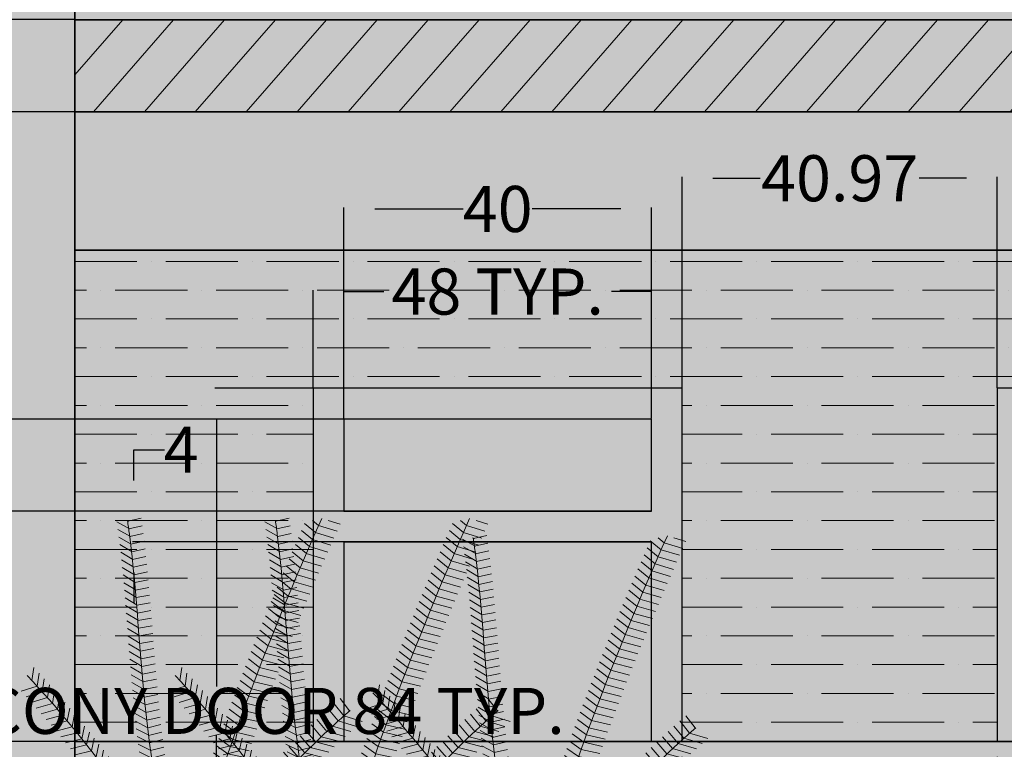
# Model space of a CAD drawing. Units: inches. Extents: x 184 to 649, y 215 to 818.
# Tile 6 of 9: x 254 to 382, y 548 to 643. Entities that reach past the tile are written whole.
import ezdxf

# ---------------------------------------------------------------- set-up
doc = ezdxf.new("R2010")
doc.units = ezdxf.units.IN
doc.header["$MEASUREMENT"] = 0
for name, color, linetype, lineweight in [('A-ANNO-DIMS', 2, 'Continuous', 18), ('A-DOOR', 4, 'Continuous', 25), ('A-ELEV', 7, 'Continuous', 35), ('A-ELEV-FILL', 9, 'Continuous', 13), ('A-ELEV-PATT', 8, 'Continuous', 13), ('L-PLNT', 84, 'Continuous', 13)]:
    doc.layers.add(name, color=color, linetype=linetype, lineweight=lineweight)
doc.styles.get("Standard").update_dxf_attribs({"font": 'arial.ttf'})
doc.dimstyles.get("Standard").update_dxf_attribs({"dimtxt": 6, "dimasz": 4, "dimexe": 0.18, "dimexo": 0.0625, "dimgap": 0.09, "dimtad": 0, "dimtih": 1, "dimtoh": 1, "dimdec": 0, "dimzin": 0, "dimdsep": 46, "dimlunit": 3, "dimtxsty": 'Standard', "dimcen": 0.09, "dimadec": 0, "dimazin": 0, "dimtfac": 1, "dimtdec": 0, "dimtofl": 0, "dimtmove": 0, "dimatfit": 3, "dimfxl": 1, "dimtolj": 1, "dimtzin": 0, "dimarcsym": 0})

# ---------------------------------------------------------------- blocks, each defined once
blk = doc.blocks.new('PLANT-PALM')
for p, q in [((274.94, 416.06), (273.31, 416.97)), ((274.8, 417.06), (274.61, 417.16)), ((274.73, 417.05), (276.46, 417.47)), ((274.87, 416.06), (276.6, 416.47)), ((299.15, 415.59), (297.73, 416.77)), ((299.55, 416.5), (298.76, 417.16)), ((299.55, 416.5), (301.94, 415.78)), ((300.78, 417.16), (302.34, 416.68)), ((275.06, 415.07), (273.44, 415.99)), ((275, 415.07), (276.73, 415.46)), ((298.74, 414.67), (297.33, 415.85)), ((299.14, 415.59), (301.53, 414.87)), ((275.18, 414.08), (273.57, 415)), ((275.3, 413.08), (273.69, 414.02)), ((275.12, 414.07), (276.85, 414.46)), ((297.95, 412.84), (296.52, 414.01)), ((298.34, 413.75), (296.92, 414.93)), ((298.34, 413.75), (300.74, 413.04)), ((298.74, 414.67), (301.13, 413.96)), ((275.4, 412.09), (273.8, 413.03)), ((275.23, 413.08), (276.97, 413.45)), ((275.34, 412.09), (277.08, 412.45)), ((297.55, 411.92), (296.12, 413.09)), ((297.94, 412.84), (300.34, 412.13)), ((275.51, 411.09), (273.9, 412.04)), ((275.44, 411.09), (277.18, 411.45)), ((296.76, 410.08), (295.33, 411.24)), ((297.16, 411), (295.73, 412.16)), ((297.55, 411.92), (299.94, 411.22)), ((275.6, 410.1), (274, 411.05)), ((275.69, 409.1), (274.1, 410.06)), ((275.54, 410.1), (277.28, 410.45)), ((296.38, 409.16), (294.94, 410.32)), ((296.76, 410.08), (299.16, 409.39)), ((297.16, 411), (299.55, 410.3)), ((275.78, 408.11), (274.19, 409.06)), ((275.63, 409.1), (277.38, 409.45)), ((295.99, 408.23), (294.55, 409.39)), ((296.37, 409.16), (298.78, 408.47)), ((275.87, 407.11), (274.28, 408.07)), ((275.72, 408.1), (277.47, 408.45)), ((275.81, 407.11), (277.55, 407.44)), ((295.22, 406.39), (293.78, 407.54)), ((295.6, 407.31), (294.16, 408.46)), ((295.99, 408.24), (298.39, 407.56)), ((275.95, 406.11), (274.36, 407.08)), ((276.03, 405.12), (274.44, 406.08)), ((275.89, 406.11), (277.64, 406.45)), ((294.84, 405.46), (293.39, 406.61)), ((295.22, 406.39), (297.62, 405.72)), ((295.6, 407.31), (298.01, 406.64)), ((276.11, 404.12), (274.52, 405.08)), ((275.97, 405.11), (277.72, 405.45)), ((294.46, 404.54), (293.01, 405.68)), ((294.84, 405.46), (297.25, 404.8)), ((276.19, 403.12), (274.6, 404.09)), ((276.05, 404.12), (277.8, 404.45)), ((293.71, 402.68), (292.26, 403.82)), ((294.08, 403.61), (292.63, 404.75)), ((294.08, 403.61), (296.49, 402.96)), ((294.46, 404.54), (296.87, 403.88)), ((276.27, 402.13), (274.68, 403.09)), ((276.13, 403.12), (277.88, 403.45)), ((276.21, 402.12), (277.96, 402.46)), ((293.34, 401.76), (291.88, 402.89)), ((293.71, 402.68), (296.12, 402.04)), ((276.35, 401.13), (274.75, 402.09)), ((276.43, 400.13), (274.83, 401.09)), ((276.29, 401.13), (278.04, 401.46)), ((292.6, 399.9), (291.14, 401.02)), ((292.97, 400.83), (291.51, 401.95)), ((293.34, 401.76), (295.75, 401.12)), ((276.51, 399.14), (274.91, 400.09)), ((276.37, 400.13), (278.12, 400.47)), ((292.24, 398.97), (290.77, 400.08)), ((292.6, 399.9), (295.02, 399.27)), ((292.97, 400.83), (295.38, 400.2)), ((276.59, 398.14), (274.99, 399.09)), ((276.45, 399.13), (278.2, 399.47)), ((276.53, 398.14), (278.28, 398.48)), ((291.87, 398.03), (290.41, 399.15)), ((292.24, 398.97), (294.65, 398.35)), ((262.25, 396.34), (262.49, 398.02)), ((262.93, 395.6), (263.18, 397.28)), ((276.67, 397.14), (275.07, 398.09)), ((276.76, 396.15), (275.15, 397.08)), ((276.62, 397.14), (278.36, 397.49)), ((291.16, 396.17), (289.68, 397.27)), ((291.51, 397.1), (290.04, 398.21)), ((291.51, 397.1), (293.94, 396.5)), ((291.87, 398.03), (294.29, 397.42)), ((263.6, 394.85), (263.86, 396.53)), ((276.84, 395.15), (275.23, 396.08)), ((276.7, 396.14), (278.45, 396.5)), ((290.8, 395.23), (289.33, 396.34)), ((291.16, 396.17), (293.58, 395.57)), ((262.93, 395.59), (260.85, 394.94)), ((263.6, 394.85), (261.51, 394.21)), ((264.26, 394.11), (264.53, 395.78)), ((264.91, 393.35), (265.2, 395.02)), ((276.94, 394.16), (275.32, 395.08)), ((276.79, 395.15), (278.54, 395.51)), ((276.89, 394.15), (278.63, 394.52)), ((290.45, 394.3), (288.97, 395.4)), ((290.8, 395.23), (293.23, 394.64)), ((264.26, 394.1), (262.17, 393.48)), ((264.92, 393.35), (262.82, 392.74)), ((265.57, 392.59), (265.86, 394.26)), ((266.21, 391.83), (266.52, 393.5)), ((277.03, 393.16), (275.41, 394.07)), ((276.99, 393.16), (278.72, 393.54)), ((289.75, 392.42), (288.27, 393.51)), ((290.1, 393.36), (288.62, 394.45)), ((290.1, 393.36), (292.53, 392.78)), ((290.45, 394.3), (292.88, 393.71)), ((302.82, 391.73), (301.57, 393.3)), ((303.57, 392.39), (302.33, 393.98)), ((265.57, 392.59), (263.47, 391.99)), ((266.85, 391.06), (267.17, 392.73)), ((277.13, 392.17), (275.5, 393.07)), ((277.24, 391.17), (275.6, 392.06)), ((277.09, 392.16), (278.82, 392.55)), ((289.41, 391.48), (287.92, 392.57)), ((289.75, 392.42), (292.18, 391.85)), ((302.08, 391.06), (300.81, 392.62)), ((266.22, 391.82), (264.11, 391.25)), ((266.86, 391.06), (264.75, 390.49)), ((267.49, 390.29), (267.81, 391.95)), ((268.12, 389.51), (268.45, 391.17)), ((277.35, 390.18), (275.71, 391.05)), ((277.19, 391.17), (278.93, 391.57)), ((288.73, 389.6), (287.23, 390.68)), ((289.07, 390.54), (287.57, 391.62)), ((289.41, 391.48), (291.84, 390.92)), ((300.61, 389.7), (299.32, 391.25)), ((301.34, 390.38), (300.06, 391.94)), ((302.08, 391.06), (304.47, 390.35)), ((302.82, 391.73), (305.21, 391)), ((267.49, 390.29), (265.38, 389.73)), ((268.12, 389.51), (266.01, 388.97)), ((268.75, 388.73), (269.09, 390.39)), ((269.37, 387.95), (269.72, 389.61)), ((277.47, 389.19), (275.82, 390.05)), ((277.31, 390.18), (279.04, 390.59)), ((277.43, 389.18), (279.15, 389.61)), ((288.39, 388.66), (286.89, 389.73)), ((288.73, 389.6), (291.16, 389.05)), ((289.07, 390.54), (291.5, 389.98)), ((299.16, 388.32), (297.85, 389.85)), ((299.88, 389.01), (298.59, 390.55)), ((300.61, 389.7), (303.01, 389.03)), ((301.34, 390.38), (303.74, 389.69)), ((268.75, 388.73), (266.64, 388.2)), ((269.99, 387.16), (270.34, 388.82)), ((277.6, 388.2), (275.94, 389.04)), ((277.56, 388.19), (279.28, 388.63)), ((288.06, 387.72), (286.56, 388.79)), ((288.39, 388.66), (290.83, 388.12)), ((297.74, 386.91), (296.41, 388.42)), ((298.45, 387.62), (297.13, 389.14)), ((299.16, 388.32), (301.58, 387.68)), ((299.88, 389.01), (302.29, 388.36)), ((269.37, 387.95), (267.26, 387.43)), ((269.99, 387.16), (267.87, 386.65)), ((270.6, 386.37), (270.97, 388.03)), ((271.21, 385.58), (271.58, 387.24)), ((277.73, 387.21), (276.06, 388.03)), ((277.87, 386.22), (276.2, 387.03)), ((277.69, 387.2), (279.41, 387.66)), ((287.4, 385.83), (285.89, 386.89)), ((287.73, 386.77), (286.22, 387.84)), ((288.06, 387.72), (290.5, 387.18)), ((296.33, 385.49), (294.99, 386.98)), ((297.03, 386.2), (295.69, 387.71)), ((297.74, 386.91), (300.16, 386.31)), ((298.45, 387.62), (300.87, 387)), ((270.61, 386.37), (268.48, 385.87)), ((271.22, 385.58), (269.09, 385.09)), ((271.82, 384.79), (272.2, 386.44)), ((272.42, 383.99), (272.8, 385.64)), ((278.02, 385.23), (276.34, 386.02)), ((277.83, 386.21), (279.55, 386.69)), ((277.99, 385.22), (279.69, 385.72)), ((287.08, 384.88), (285.56, 385.94)), ((287.4, 385.83), (289.84, 385.31)), ((287.73, 386.77), (290.17, 386.25)), ((295.64, 384.77), (294.28, 386.26)), ((297.03, 386.2), (299.46, 385.61)), ((271.82, 384.79), (269.7, 384.3)), ((273.02, 383.19), (273.41, 384.84)), ((278.18, 384.24), (276.49, 385.01)), ((278.15, 384.24), (279.85, 384.75)), ((286.76, 383.94), (285.24, 384.98)), ((287.08, 384.88), (289.52, 384.37)), ((294.26, 383.32), (292.89, 384.79)), ((294.95, 384.05), (293.58, 385.53)), ((295.64, 384.77), (298.07, 384.21)), ((296.33, 385.49), (298.76, 384.92)), ((272.43, 383.99), (270.3, 383.51)), ((273.03, 383.19), (270.9, 382.72)), ((273.62, 382.39), (274.01, 384.04)), ((274.21, 381.58), (274.61, 383.23)), ((278.36, 383.26), (276.65, 384)), ((278.54, 382.28), (276.83, 382.99)), ((278.32, 383.25), (280.02, 383.79)), ((286.12, 382.04), (284.6, 383.08)), ((286.44, 382.99), (284.92, 384.03)), ((286.75, 383.94), (289.2, 383.43)), ((292.9, 381.85), (291.51, 383.31)), ((293.58, 382.59), (292.2, 384.05)), ((294.26, 383.32), (296.7, 382.79)), ((294.95, 384.05), (297.38, 383.5)), ((273.62, 382.39), (271.49, 381.93)), ((274.8, 380.78), (275.21, 382.42)), ((278.74, 381.3), (277.01, 381.99)), ((278.51, 382.27), (280.2, 382.83)), ((278.71, 381.29), (280.39, 381.87)), ((285.81, 381.09), (284.28, 382.12)), ((286.12, 382.04), (288.57, 381.55)), ((286.44, 382.99), (288.88, 382.49)), ((291.56, 380.37), (290.15, 381.81)), ((292.23, 381.11), (290.83, 382.56)), ((292.9, 381.85), (295.35, 381.35)), ((293.58, 382.59), (296.02, 382.07)), ((274.22, 381.58), (272.09, 381.13)), ((274.81, 380.78), (272.68, 380.33)), ((275.39, 379.97), (275.8, 381.61)), ((275.98, 379.16), (276.39, 380.8)), ((278.95, 380.32), (277.21, 380.98)), ((278.92, 380.31), (280.59, 380.92)), ((285.5, 380.14), (283.97, 381.16)), ((285.81, 381.09), (288.26, 380.61)), ((290.9, 379.63), (289.48, 381.06)), ((292.23, 381.11), (294.68, 380.62)), ((275.4, 379.97), (273.26, 379.53)), ((275.99, 379.16), (273.85, 378.72)), ((276.56, 378.35), (276.98, 379.99)), ((277.14, 377.53), (277.56, 379.18)), ((279.17, 379.35), (277.42, 379.97)), ((279.15, 379.34), (280.81, 379.98)), ((284.9, 378.23), (283.36, 379.24)), ((285.2, 379.18), (283.66, 380.2)), ((285.2, 379.18), (287.65, 378.72)), ((285.5, 380.14), (287.95, 379.67)), ((289.58, 378.12), (288.15, 379.54)), ((290.23, 378.87), (288.81, 380.3)), ((290.9, 379.63), (293.35, 379.16)), ((291.56, 380.37), (294.01, 379.89)), ((276.57, 378.35), (274.43, 377.92)), ((279.41, 378.38), (277.65, 378.97)), ((277.72, 376.72), (278.15, 378.36)), ((279.67, 377.41), (277.9, 377.96)), ((279.39, 378.37), (281.04, 379.04)), ((279.65, 377.4), (281.29, 378.11)), ((284.6, 377.27), (283.06, 378.28)), ((284.9, 378.23), (287.35, 377.78)), ((288.27, 376.61), (286.83, 378.01)), ((288.92, 377.36), (287.49, 378.78)), ((289.58, 378.12), (292.03, 377.67)), ((290.23, 378.87), (292.69, 378.42)), ((277.15, 377.53), (275.02, 377.11)), ((277.74, 376.72), (275.6, 376.3)), ((279.95, 376.45), (278.16, 376.96)), ((278.3, 375.9), (278.73, 377.55)), ((278.88, 375.09), (279.31, 376.73)), ((279.93, 376.44), (281.55, 377.18)), ((284.31, 376.32), (282.76, 377.32)), ((284.6, 377.28), (287.06, 376.83)), ((287.63, 375.84), (286.18, 377.24)), ((288.27, 376.61), (290.73, 376.18)), ((288.92, 377.36), (291.38, 376.93)), ((278.31, 375.91), (276.18, 375.49)), ((280.24, 375.49), (278.44, 375.96)), ((279.46, 374.27), (279.88, 375.91)), ((280.23, 375.49), (281.83, 376.27)), ((280.55, 374.54), (282.13, 375.36)), ((283.73, 374.4), (282.18, 375.39)), ((284.02, 375.36), (282.47, 376.36)), ((284.02, 375.36), (286.48, 374.94)), ((284.31, 376.32), (286.77, 375.89)), ((286.34, 374.31), (284.89, 375.7)), ((286.98, 375.08), (285.53, 376.47)), ((287.63, 375.84), (290.09, 375.43)), ((278.89, 375.09), (276.75, 374.67)), ((279.47, 374.27), (277.33, 373.86)), ((280.56, 374.55), (278.75, 374.97)), ((280.03, 373.45), (280.46, 375.09)), ((280.61, 372.64), (281.04, 374.28)), ((280.89, 373.6), (282.45, 374.46)), ((283.45, 373.44), (281.89, 374.43)), ((285.07, 372.76), (283.61, 374.14)), ((283.73, 374.4), (286.2, 373.99)), ((285.71, 373.54), (284.24, 374.92)), ((286.34, 374.31), (288.81, 373.91)), ((286.98, 375.08), (289.45, 374.67)), ((280.05, 373.46), (277.91, 373.04)), ((280.9, 373.61), (279.08, 373.97)), ((281.26, 372.67), (279.43, 372.98)), ((281.18, 371.82), (281.61, 373.46)), ((281.26, 372.67), (282.79, 373.58)), ((283.18, 372.48), (281.61, 373.46)), ((284.44, 371.99), (282.97, 373.36)), ((283.45, 373.44), (285.92, 373.04)), ((285.07, 372.76), (287.54, 372.39)), ((285.71, 373.54), (288.17, 373.15)), ((280.62, 372.64), (278.48, 372.23)), ((281.2, 371.82), (279.05, 371.41)), ((281.65, 371.75), (279.81, 372)), ((282.9, 371.52), (281.33, 372.49)), ((281.65, 371.75), (283.15, 372.7)), ((281.77, 371), (282.24, 372.12)), ((282.07, 370.84), (283.54, 371.85)), ((282.9, 371.52), (285.37, 371.14)), ((283.18, 372.48), (285.64, 372.09)), ((284.44, 371.99), (286.91, 371.62)), ((281.77, 371), (279.63, 370.59)), ((282.63, 370.56), (285.1, 370.19))]:
    blk.add_line(p, q)
blk.add_open_spline([(274.68, 417.16), (274.77, 416.57), (276.95, 400.47), (276.36, 381.5), (282.64, 369.73)], degree=3, knots=[87.299959, 87.299959, 87.299959, 87.299959, 88.780677, 127.704389, 127.704389, 127.704389, 127.704389])
for points in [[(282.63, 370.56), (286.61, 384.99), (292.84, 401.43), (299.95, 417.41)], [(282.55, 369.88), (275.93, 379.33), (269.31, 388.78), (261.65, 396.98)], [(282.64, 369.73), (290.67, 379.89), (297.61, 387.15), (303.65, 392.43)]]:
    blk.add_open_spline(points, degree=3)
blk = doc.blocks.new('DOOR-BALCONY')
for points in [[(340, 548.73), (340, 594.73), (292, 594.73), (292, 548.73)], [(336, 578.73), (336, 590.73), (296, 590.73), (296, 578.73)], [(296, 574.73), (296, 548.73)], [(336, 548.73), (336, 574.73)], [(292, 546.73), (292, 510.73), (340, 510.73), (340, 546.73)]]:
    blk.add_lwpolyline(points)
blk = doc.blocks.new('*D7')
at = {"layer": 'A-ANNO-DIMS', "color": 0, "lineweight": -2, "transparency": 16777216}
for p, q in [((291.94, 594.73), (279.22, 594.73)), ((279.4, 590.73), (279.4, 555.92)), ((279.4, 514.73), (279.4, 549.53)), ((291.94, 510.73), (279.22, 510.73))]:
    blk.add_line(p, q, dxfattribs=at)
at = {"layer": 'A-ANNO-DIMS', "color": 0, "transparency": 16777216}
for points in [[(278.73, 590.73), (280.07, 590.73), (279.4, 594.73)], [(278.73, 514.73), (280.07, 514.73), (279.4, 510.73)]]:
    blk.add_solid(points, dxfattribs=at)
at = {"layer": 'Defpoints', "color": 0, "transparency": 16777216}
for p in [(279.4, 594.73), (292, 594.73), (292, 510.73)]:
    blk.add_point(p, dxfattribs=at)
at = {"layer": 'A-ANNO-DIMS', "color": 0, "transparency": 16777216, "insert": (279.4, 552.73), "char_height": 6, "attachment_point": 5}
blk.add_mtext('\\A1;BALCONY DOOR 84 TYP.', dxfattribs=at)
blk = doc.blocks.new('*D8')
at = {"layer": 'A-ANNO-DIMS', "color": 0, "lineweight": -2, "transparency": 16777216}
for p, q in [((292, 594.79), (292, 607.51)), ((296, 607.33), (301.19, 607.33)), ((336, 607.33), (330.81, 607.33)), ((340, 594.79), (340, 607.51))]:
    blk.add_line(p, q, dxfattribs=at)
at = {"layer": 'A-ANNO-DIMS', "color": 0, "transparency": 16777216}
for points in [[(296, 607.99), (296, 606.66), (292, 607.33)], [(336, 607.99), (336, 606.66), (340, 607.33)]]:
    blk.add_solid(points, dxfattribs=at)
at = {"layer": 'Defpoints', "color": 0, "transparency": 16777216}
for p in [(340, 607.33), (292, 594.73), (340, 594.73)]:
    blk.add_point(p, dxfattribs=at)
at = {"layer": 'A-ANNO-DIMS', "color": 0, "transparency": 16777216, "insert": (316, 607.33), "char_height": 6, "attachment_point": 5}
blk.add_mtext('\\A1;48 TYP.', dxfattribs=at)
blk = doc.blocks.new('*D37')
at = {"layer": 'A-ANNO-DIMS', "color": 0, "lineweight": -2, "transparency": 16777216}
for p, q in [((260.91, 548.73), (196.12, 548.73)), ((196.3, 544.73), (196.3, 532.88)), ((196.3, 514.73), (196.3, 526.57)), ((260.91, 510.73), (196.12, 510.73))]:
    blk.add_line(p, q, dxfattribs=at)
at = {"layer": 'A-ANNO-DIMS', "color": 0, "transparency": 16777216}
for points in [[(195.63, 544.73), (196.96, 544.73), (196.3, 548.73)], [(195.63, 514.73), (196.96, 514.73), (196.3, 510.73)]]:
    blk.add_solid(points, dxfattribs=at)
at = {"layer": 'Defpoints', "color": 0, "transparency": 16777216}
for p in [(196.3, 548.73), (260.97, 548.73), (260.97, 510.73)]:
    blk.add_point(p, dxfattribs=at)
at = {"layer": 'A-ANNO-DIMS', "color": 0, "transparency": 16777216, "insert": (196.3, 529.73), "char_height": 6, "attachment_point": 5}
blk.add_mtext('\\A1;38', dxfattribs=at)
blk = doc.blocks.new('*D38')
at = {"layer": 'A-ANNO-DIMS', "color": 0, "lineweight": -2, "transparency": 16777216}
for p, q in [((260.91, 630.73), (196.12, 630.73)), ((196.3, 626.73), (196.3, 592.88)), ((196.3, 552.73), (196.3, 586.57)), ((260.91, 548.73), (196.12, 548.73))]:
    blk.add_line(p, q, dxfattribs=at)
at = {"layer": 'A-ANNO-DIMS', "color": 0, "transparency": 16777216}
for points in [[(195.63, 626.73), (196.96, 626.73), (196.3, 630.73)], [(195.63, 552.73), (196.96, 552.73), (196.3, 548.73)]]:
    blk.add_solid(points, dxfattribs=at)
at = {"layer": 'Defpoints', "color": 0, "transparency": 16777216}
for p in [(196.3, 630.73), (260.97, 630.73), (260.97, 548.73)]:
    blk.add_point(p, dxfattribs=at)
at = {"layer": 'A-ANNO-DIMS', "color": 0, "transparency": 16777216, "insert": (196.3, 589.73), "char_height": 6, "attachment_point": 5}
blk.add_mtext('\\A1;82', dxfattribs=at)
blk = doc.blocks.new('*D39')
at = {"layer": 'A-ANNO-DIMS', "color": 0, "lineweight": -2, "transparency": 16777216}
for p, q in [((196.3, 642.73), (196.3, 646.73)), ((196.3, 646.73), (200.3, 646.73)), ((260.91, 642.73), (196.12, 642.73)), ((196.3, 634.73), (196.3, 638.73)), ((260.91, 630.73), (196.12, 630.73))]:
    blk.add_line(p, q, dxfattribs=at)
at = {"layer": 'A-ANNO-DIMS', "color": 0, "transparency": 16777216}
for points in [[(195.63, 638.73), (196.96, 638.73), (196.3, 642.73)], [(195.63, 634.73), (196.96, 634.73), (196.3, 630.73)]]:
    blk.add_solid(points, dxfattribs=at)
at = {"layer": 'Defpoints', "color": 0, "transparency": 16777216}
for p in [(196.3, 642.73), (260.97, 642.73), (260.97, 630.73)]:
    blk.add_point(p, dxfattribs=at)
at = {"layer": 'A-ANNO-DIMS', "color": 0, "transparency": 16777216, "insert": (204.37, 646.73), "char_height": 6, "attachment_point": 5}
blk.add_mtext('\\A1;12', dxfattribs=at)
blk = doc.blocks.new('*D59')
at = {"layer": 'A-ANNO-DIMS', "color": 0, "lineweight": -2, "transparency": 16777216}
for p, q in [((340, 594.79), (340, 622.26)), ((344, 622.08), (350.15, 622.08)), ((376.97, 622.08), (370.82, 622.08)), ((380.97, 594.79), (380.97, 622.26))]:
    blk.add_line(p, q, dxfattribs=at)
at = {"layer": 'A-ANNO-DIMS', "color": 0, "transparency": 16777216}
for points in [[(344, 622.74), (344, 621.41), (340, 622.08)], [(376.97, 622.74), (376.97, 621.41), (380.97, 622.08)]]:
    blk.add_solid(points, dxfattribs=at)
at = {"layer": 'Defpoints', "color": 0, "transparency": 16777216}
for p in [(380.97, 622.08), (340, 594.73), (380.97, 594.73)]:
    blk.add_point(p, dxfattribs=at)
at = {"layer": 'A-ANNO-DIMS', "color": 0, "transparency": 16777216, "insert": (360.49, 622.08), "char_height": 6, "attachment_point": 5}
blk.add_mtext('\\A1;40.97', dxfattribs=at)
blk = doc.blocks.new('*D60')
at = {"layer": 'A-ANNO-DIMS', "color": 0, "lineweight": -2, "transparency": 16777216}
for p, q in [((296, 590.79), (296, 618.26)), ((300, 618.08), (311.5, 618.08)), ((332, 618.08), (320.5, 618.08)), ((336, 590.79), (336, 618.26))]:
    blk.add_line(p, q, dxfattribs=at)
at = {"layer": 'A-ANNO-DIMS', "color": 0, "transparency": 16777216}
for points in [[(300, 618.74), (300, 617.41), (296, 618.08)], [(332, 618.74), (332, 617.41), (336, 618.08)]]:
    blk.add_solid(points, dxfattribs=at)
at = {"layer": 'Defpoints', "color": 0, "transparency": 16777216}
for p in [(336, 618.08), (296, 590.73), (336, 590.73)]:
    blk.add_point(p, dxfattribs=at)
at = {"layer": 'A-ANNO-DIMS', "color": 0, "transparency": 16777216, "insert": (316, 618.08), "char_height": 6, "attachment_point": 5}
blk.add_mtext('\\A1;40', dxfattribs=at)
blk = doc.blocks.new('*D61')
at = {"layer": 'A-ANNO-DIMS', "color": 0, "lineweight": -2, "transparency": 16777216}
for p, q in [((196.3, 590.73), (196.3, 594.73)), ((196.3, 594.73), (200.3, 594.73)), ((295.94, 590.73), (196.12, 590.73)), ((196.3, 582.73), (196.3, 586.73)), ((295.94, 578.73), (196.12, 578.73))]:
    blk.add_line(p, q, dxfattribs=at)
at = {"layer": 'A-ANNO-DIMS', "color": 0, "transparency": 16777216}
for points in [[(195.63, 586.73), (196.96, 586.73), (196.3, 590.73)], [(195.63, 582.73), (196.96, 582.73), (196.3, 578.73)]]:
    blk.add_solid(points, dxfattribs=at)
at = {"layer": 'Defpoints', "color": 0, "transparency": 16777216}
for p in [(196.3, 590.73), (296, 590.73), (296, 578.73)]:
    blk.add_point(p, dxfattribs=at)
at = {"layer": 'A-ANNO-DIMS', "color": 0, "transparency": 16777216, "insert": (204.37, 594.73), "char_height": 6, "attachment_point": 5}
blk.add_mtext('\\A1;12', dxfattribs=at)
blk = doc.blocks.new('*D62')
at = {"layer": 'A-ANNO-DIMS', "color": 0, "lineweight": -2, "transparency": 16777216}
for p, q in [((268.65, 582.73), (268.65, 586.73)), ((268.65, 586.73), (272.65, 586.73)), ((295.94, 578.73), (268.47, 578.73)), ((295.94, 574.73), (268.47, 574.73)), ((268.65, 570.73), (268.65, 566.73))]:
    blk.add_line(p, q, dxfattribs=at)
at = {"layer": 'A-ANNO-DIMS', "color": 0, "transparency": 16777216}
for points in [[(267.98, 582.73), (269.32, 582.73), (268.65, 578.73)], [(267.98, 570.73), (269.32, 570.73), (268.65, 574.73)]]:
    blk.add_solid(points, dxfattribs=at)
at = {"layer": 'Defpoints', "color": 0, "transparency": 16777216}
for p in [(268.65, 578.73), (296, 578.73), (296, 574.73)]:
    blk.add_point(p, dxfattribs=at)
at = {"layer": 'A-ANNO-DIMS', "color": 0, "transparency": 16777216, "insert": (274.81, 586.73), "char_height": 6, "attachment_point": 5}
blk.add_mtext('\\A1;4', dxfattribs=at)

msp = doc.modelspace()

# ---------------------------------------------------------------- hatches: boundary and pattern name
at = {"layer": 'A-ELEV-FILL'}
h = msp.add_hatch(color=256, dxfattribs=at)
h.dxf.hatch_style = 1
h.paths.add_polyline_path([(452.9726, 369.7265), (248.9726, 369.7265), (248.9726, 246.7265), (275.9726, 246.7265), (275.9726, 328.7265), (437.9726, 328.7265), (437.9726, 246.7265), (446.6666, 246.7265), (452.9726, 282.7265)])
h.paths.add_polyline_path([(275.9726, 340.7265), (275.9726, 354.7265), (437.9726, 354.7265), (437.9726, 340.7265)], flags=16)
h.paths.add_polyline_path([(452.9726, 510.7265), (260.9726, 510.7265), (260.9726, 642.7265), (260.9726, 699.7265), (367.0226, 699.7265), (373.9381, 706.7265), (260.9726, 706.7265), (260.9726, 715.7265), (382.8295, 715.7265), (389.745, 722.7265), (260.9726, 722.7265), (260.9726, 731.7265), (398.6364, 731.7265), (405.5519, 738.7265), (260.9726, 738.7265), (260.9726, 747.7265), (414.4433, 747.7265), (421.3588, 754.7265), (260.9726, 754.7265), (260.9726, 763.7265), (430.2502, 763.7265), (437.1657, 770.7265), (260.9726, 770.7265), (260.9726, 779.7265), (446.057, 779.7265), (452.9726, 786.7265), (248.9726, 786.7265), (248.9726, 369.7265), (260.9726, 369.7265), (260.9726, 498.7265), (452.9726, 498.7265)])
h = msp.add_hatch(color=256, dxfattribs=at)
h.dxf.hatch_style = 1
h.paths.add_polyline_path([(452.9726, 654.7265), (260.9726, 654.7265), (260.9726, 642.7265), (452.9726, 642.7265)])
h = msp.add_hatch(color=256, dxfattribs=at)
h.dxf.hatch_style = 1
h.paths.add_polyline_path([(440.9726, 630.7265), (260.9726, 630.7265), (260.9726, 612.7265), (422.9726, 612.7265), (422.9726, 594.7265), (428.9726, 594.7265), (428.9726, 548.7265), (440.9726, 548.7265)])
h.paths.add_polyline_path([(452.9726, 642.7265), (440.9726, 630.7265), (440.9726, 548.7265), (452.9726, 548.7265)])
h = msp.add_hatch(color=256, dxfattribs=at)
h.dxf.hatch_style = 1
h.paths.add_polyline_path([(452.9726, 642.7265), (260.9726, 642.7265), (260.9726, 630.7265), (440.9726, 630.7265)])
h = msp.add_hatch(color=256, dxfattribs=at)
h.dxf.hatch_style = 1
h.paths.add_polyline_path([(380.9726, 594.7265), (422.9726, 594.7265), (422.9726, 612.7265), (260.9726, 612.7265), (260.9726, 548.7265), (291.9998, 548.7265), (291.9998, 594.7265), (339.9998, 594.7265), (339.9998, 548.7265), (380.9726, 548.7265)])
h = msp.add_hatch(color=256, dxfattribs=at)
h.dxf.hatch_style = 1
h.paths.add_polyline_path([(339.9998, 594.7265), (291.9998, 594.7265), (291.9998, 548.7265), (295.9998, 548.7265), (295.9998, 574.7265), (335.9998, 574.7265), (335.9998, 548.7265), (339.9998, 548.7265)])
h.paths.add_polyline_path([(335.9998, 578.7265), (295.9998, 578.7265), (295.9998, 590.7265), (335.9998, 590.7265)], flags=16)
h.paths.add_polyline_path([(422.9726, 578.7265), (384.9726, 578.7265), (384.9726, 590.7265), (422.9726, 590.7265), (422.9726, 594.7265), (380.9726, 594.7265), (380.9726, 548.7265), (384.9726, 548.7265), (384.9726, 574.7265), (422.9726, 574.7265)])
h = msp.add_hatch(color=256, dxfattribs=at)
h.dxf.hatch_style = 1
h.paths.add_polyline_path([(335.9998, 433.5037), (295.9998, 433.5037), (295.9998, 369.7265), (335.9998, 369.7265)])
h.paths.add_polyline_path([(335.9998, 449.5037), (295.9998, 449.5037), (295.9998, 437.5037), (335.9998, 437.5037)])
h.paths.add_polyline_path([(422.2268, 449.5037), (384.9726, 449.5037), (384.9726, 437.5037), (422.2268, 437.5037)])
h.paths.add_polyline_path([(422.2268, 433.5037), (384.9726, 433.5037), (384.9726, 369.7265), (422.2268, 369.7265)])
h.paths.add_polyline_path([(335.9998, 590.7265), (295.9998, 590.7265), (295.9998, 578.7265), (335.9998, 578.7265)])
h.paths.add_polyline_path([(335.9998, 574.7265), (295.9998, 574.7265), (295.9998, 548.7265), (335.9998, 548.7265)])
h.paths.add_polyline_path([(422.9726, 590.7265), (384.9726, 590.7265), (384.9726, 578.7265), (422.9726, 578.7265)])
h.paths.add_polyline_path([(422.9726, 574.7265), (384.9726, 574.7265), (384.9726, 548.7265), (422.9726, 548.7265)])
h = msp.add_hatch(color=256, dxfattribs=at)
h.dxf.hatch_style = 1
h.paths.add_polyline_path([(452.9726, 548.7265), (260.9726, 548.7265), (260.9726, 546.7265), (452.9726, 546.7265)])
h.paths.add_polyline_path([(262.9726, 546.7265), (260.9726, 546.7265), (260.9726, 510.7265), (262.9726, 510.7265)])
h.paths.add_polyline_path([(269.3864, 546.7265), (267.3864, 546.7265), (267.3864, 510.7265), (269.3864, 510.7265)])
h.paths.add_polyline_path([(275.8001, 546.7265), (273.8001, 546.7265), (273.8001, 510.7265), (275.8001, 510.7265)])
h.paths.add_polyline_path([(282.2139, 546.7265), (280.2139, 546.7265), (280.2139, 510.7265), (282.2139, 510.7265)])
h.paths.add_polyline_path([(288.6277, 546.7265), (286.6277, 546.7265), (286.6277, 510.7265), (288.6277, 510.7265)])
h.paths.add_polyline_path([(295.0415, 546.7265), (293.0415, 546.7265), (293.0415, 510.7265), (295.0415, 510.7265)])
h.paths.add_polyline_path([(301.4553, 546.7265), (299.4553, 546.7265), (299.4553, 514.7265), (301.4553, 514.7265)])
h.paths.add_polyline_path([(307.8691, 546.7265), (305.8691, 546.7265), (305.8691, 514.7265), (307.8691, 514.7265)])
h.paths.add_polyline_path([(314.2829, 546.7265), (312.2829, 546.7265), (312.2829, 514.7265), (314.2829, 514.7265)])
h.paths.add_polyline_path([(320.6967, 546.7265), (318.6967, 546.7265), (318.6967, 514.7265), (320.6967, 514.7265)])
h.paths.add_polyline_path([(327.1105, 546.7265), (325.1105, 546.7265), (325.1105, 514.7265), (327.1105, 514.7265)])
h.paths.add_polyline_path([(333.5243, 546.7265), (331.5243, 546.7265), (331.5243, 514.7265), (333.5243, 514.7265)])
h.paths.add_polyline_path([(339.9381, 546.7265), (337.9381, 546.7265), (337.9381, 510.7265), (339.9381, 510.7265)])
h.paths.add_polyline_path([(346.3519, 546.7265), (344.3519, 546.7265), (344.3519, 510.7265), (346.3519, 510.7265)])
h.paths.add_polyline_path([(352.7657, 546.7265), (350.7657, 546.7265), (350.7657, 510.7265), (352.7657, 510.7265)])
h.paths.add_polyline_path([(359.1795, 546.7265), (357.1795, 546.7265), (357.1795, 510.7265), (359.1795, 510.7265)])
h.paths.add_polyline_path([(365.5932, 546.7265), (363.5932, 546.7265), (363.5932, 510.7265), (365.5932, 510.7265)])
h.paths.add_polyline_path([(372.007, 546.7265), (370.007, 546.7265), (370.007, 510.7265), (372.007, 510.7265)])
h.paths.add_polyline_path([(378.4208, 546.7265), (376.4208, 546.7265), (376.4208, 510.7265), (378.4208, 510.7265)])
h.paths.add_polyline_path([(384.8346, 546.7265), (382.8346, 546.7265), (382.8346, 510.7265), (384.8346, 510.7265)])
h.paths.add_polyline_path([(391.2484, 546.7265), (389.2484, 546.7265), (389.2484, 514.7265), (391.2484, 514.7265)])
h.paths.add_polyline_path([(397.6622, 546.7265), (395.6622, 546.7265), (395.6622, 514.7265), (397.6622, 514.7265)])
h.paths.add_polyline_path([(404.076, 546.7265), (402.076, 546.7265), (402.076, 514.7265), (404.076, 514.7265)])
h.paths.add_polyline_path([(410.4898, 546.7265), (408.4898, 546.7265), (408.4898, 514.7265), (410.4898, 514.7265)])
h.paths.add_polyline_path([(416.9036, 546.7265), (414.9036, 546.7265), (414.9036, 514.7265), (416.9036, 514.7265)])
h.paths.add_polyline_path([(423.3174, 546.7265), (421.3174, 546.7265), (421.3174, 514.7265), (423.3174, 514.7265)])
h.paths.add_polyline_path([(423.3174, 514.7265), (421.3174, 514.7265), (421.3174, 510.7265), (423.3174, 510.7265)])
h.paths.add_polyline_path([(416.9036, 514.7265), (414.9036, 514.7265), (414.9036, 510.7265), (416.9036, 510.7265)])
h.paths.add_polyline_path([(410.4898, 514.7265), (408.4898, 514.7265), (408.4898, 510.7265), (410.4898, 510.7265)])
h.paths.add_polyline_path([(404.076, 514.7265), (402.076, 514.7265), (402.076, 510.7265), (404.076, 510.7265)])
h.paths.add_polyline_path([(397.6622, 514.7265), (395.6622, 514.7265), (395.6622, 510.7265), (397.6622, 510.7265)])
h.paths.add_polyline_path([(391.2484, 514.7265), (389.2484, 514.7265), (389.2484, 510.7265), (391.2484, 510.7265)])
h.paths.add_polyline_path([(448.9726, 546.7265), (446.9726, 546.7265), (446.9726, 510.7265), (448.9726, 510.7265)])
h.paths.add_polyline_path([(442.5588, 546.7265), (440.5588, 546.7265), (440.5588, 510.7265), (442.5588, 510.7265)])
h.paths.add_polyline_path([(436.145, 546.7265), (434.145, 546.7265), (434.145, 510.7265), (436.145, 510.7265)])
h.paths.add_polyline_path([(429.7312, 546.7265), (428.9726, 546.7265), (428.9726, 510.7265), (429.7312, 510.7265)])
h.paths.add_polyline_path([(301.4553, 514.7265), (299.4553, 514.7265), (299.4553, 510.7265), (301.4553, 510.7265)])
h.paths.add_polyline_path([(307.8691, 514.7265), (305.8691, 514.7265), (305.8691, 510.7265), (307.8691, 510.7265)])
h.paths.add_polyline_path([(314.2829, 514.7265), (312.2829, 514.7265), (312.2829, 510.7265), (314.2829, 510.7265)])
h.paths.add_polyline_path([(320.6967, 514.7265), (318.6967, 514.7265), (318.6967, 510.7265), (320.6967, 510.7265)])
h.paths.add_polyline_path([(327.1105, 514.7265), (325.1105, 514.7265), (325.1105, 510.7265), (327.1105, 510.7265)])
h.paths.add_polyline_path([(333.5243, 514.7265), (331.5243, 514.7265), (331.5243, 510.7265), (333.5243, 510.7265)])
at = {"layer": 'A-ELEV-PATT'}
h = msp.add_hatch(dxfattribs=at)
h.set_pattern_fill('ANSI31', color=256, scale=40, angle=4)
h.paths.add_polyline_path([(452.9726, 642.7265), (260.9726, 642.7265), (260.9726, 630.7265), (440.9726, 630.7265)])
h = msp.add_hatch(dxfattribs=at)
h.set_pattern_fill('ANSI36', color=256, scale=30, angle=135)
h.paths.add_polyline_path([(380.9726, 594.7265), (422.9726, 594.7265), (422.9726, 612.7265), (260.9726, 612.7265), (260.9726, 548.7265), (291.9998, 548.7265), (291.9998, 594.7265), (339.9998, 594.7265), (339.9998, 548.7265), (380.9726, 548.7265)])

# ---------------------------------------------------------------- linework, layer by layer
at = {"layer": 'A-ELEV'}
for p, q in [((260.9726, 699.7265), (260.9726, 642.7265)), ((260.9726, 642.7265), (260.9726, 510.7265)), ((452.9726, 642.7265), (260.9726, 642.7265)), ((440.9726, 630.7265), (260.9726, 630.7265)), ((422.9726, 612.7265), (260.9726, 612.7265)), ((295.9998, 578.7265), (335.9998, 578.7265)), ((335.9998, 574.7265), (295.9998, 574.7265)), ((452.9726, 548.7265), (260.9726, 548.7265))]:
    msp.add_line(p, q, dxfattribs=at)

# ---------------------------------------------------------------- block references
at = {"layer": 'A-DOOR'}
for p in [(0, 0), (88.9728, 0)]:
    msp.add_blockref('DOOR-BALCONY', p, dxfattribs=at)
at = {"layer": 'L-PLNT'}
for p in [(-6.8456, 160.3643), (12.3958, 160.3643), (38.1219, 158.1152)]:
    msp.add_blockref('PLANT-PALM', p, dxfattribs=at)

# ---------------------------------------------------------------- dimensions: what is measured, and where the dimension line sits
at = {"layer": 'A-ANNO-DIMS'}
for base, p1, p2, angle, override, picture, middle in [((196.2971, 642.7265), (260.9726, 630.7265), (260.9726, 642.7265), 90, {"dimdec": 0, "dimlfac": 1, "dimrnd": 0, "dimzin": 0, "dimdsep": 46, "dimlunit": 2}, '*D39', (204.3714, 646.7265)), ((196.2971, 630.7265), (260.9726, 548.7265), (260.9726, 630.7265), 90, {"dimdec": 0, "dimlfac": 1, "dimrnd": 0, "dimzin": 0, "dimdsep": 46, "dimlunit": 2}, '*D38', (196.2971, 589.7265)), ((380.9726, 622.0765), (339.9998, 594.7265), (380.9726, 594.7265), 0, {"dimdec": 2, "dimlfac": 1, "dimrnd": 0, "dimzin": 0, "dimdsep": 46, "dimlunit": 2}, '*D59', (360.4862, 622.0765)), ((196.2971, 590.7265), (295.9998, 578.7265), (295.9998, 590.7265), 90, {"dimdec": 0, "dimlfac": 1, "dimrnd": 0, "dimzin": 0, "dimdsep": 46, "dimlunit": 2}, '*D61', (204.3714, 594.7265)), ((268.6498, 578.7265), (295.9998, 574.7265), (295.9998, 578.7265), 90, {"dimdec": 0, "dimlfac": 1, "dimrnd": 0, "dimzin": 0, "dimdsep": 46, "dimlunit": 2}, '*D62', (274.8148, 586.7265)), ((196.2971, 548.7265), (260.9726, 510.7265), (260.9726, 548.7265), 90, {"dimdec": 0, "dimlfac": 1, "dimrnd": 0, "dimzin": 0, "dimdsep": 46, "dimlunit": 2}, '*D37', (196.2971, 529.7265))]:
    dim = msp.add_linear_dim(base=base, p1=p1, p2=p2, angle=angle, dimstyle='Standard', override=override, dxfattribs=at)
    dim.commit()
    dim.dimension.update_dxf_attribs({"geometry": picture, "text_midpoint": middle})
dim = msp.add_linear_dim(base=(335.9998, 618.0765), p1=(295.9998, 590.7265), p2=(335.9998, 590.7265), dimstyle='Standard', override={"dimdec": 0, "dimlfac": 1, "dimrnd": 0, "dimzin": 0, "dimdsep": 46, "dimlunit": 2}, dxfattribs=at)
dim.commit()
dim.dimension.update_dxf_attribs({"geometry": '*D60', "text_midpoint": (315.9998, 618.0765)})
dim = msp.add_linear_dim(base=(339.9998, 607.3265), p1=(291.9998, 594.7265), p2=(339.9998, 594.7265), text='<> TYP.', dimstyle='Standard', override={"dimdec": 0, "dimrnd": 0, "dimzin": 0, "dimlunit": 2}, dxfattribs=at)
dim.commit()
dim.dimension.update_dxf_attribs({"geometry": '*D8', "text_midpoint": (315.9998, 607.3265)})
dim = msp.add_linear_dim(base=(279.3998, 594.7265), p1=(291.9998, 510.7265), p2=(291.9998, 594.7265), angle=90, text='BALCONY DOOR <> TYP.', dimstyle='Standard', override={"dimdec": 0, "dimrnd": 0, "dimzin": 0, "dimlunit": 2}, dxfattribs=at)
dim.commit()
dim.dimension.update_dxf_attribs({"geometry": '*D7', "text_midpoint": (279.3998, 552.7265)})

doc.saveas('drawing.dxf')
